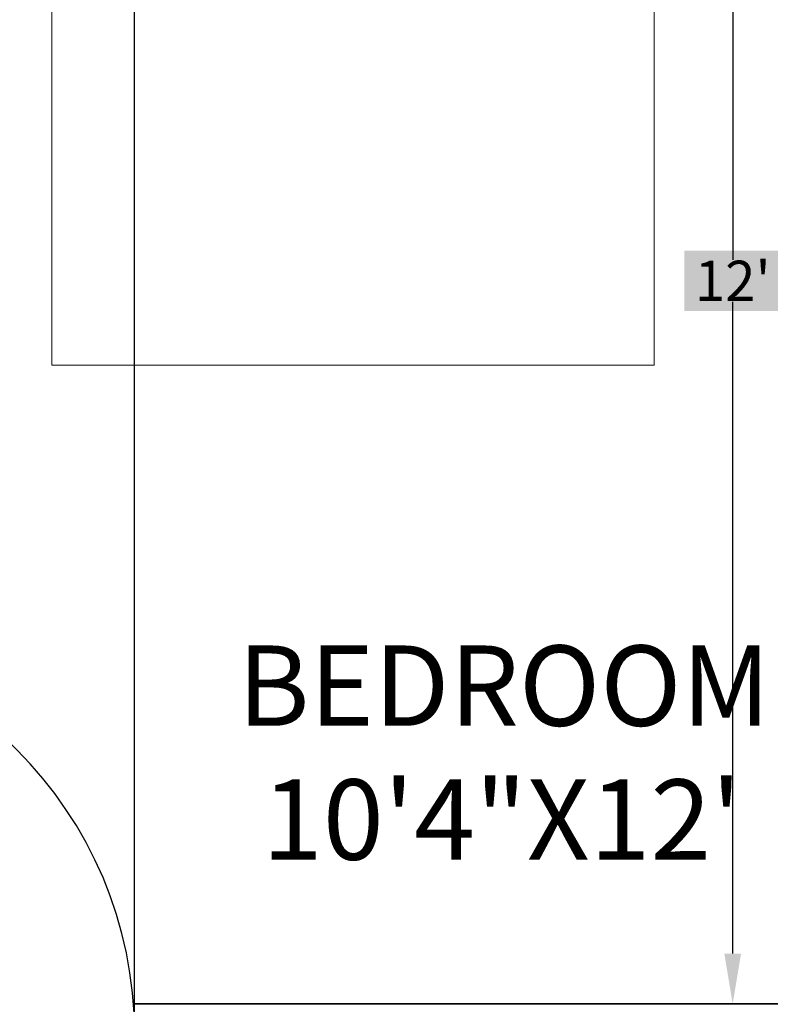
# Model space of a CAD drawing. Units: inches. Extents: x -128 to 854, y -395 to 398.
# Tile 44 of 61: x 209 to 284, y 196 to 294. Entities that reach past the tile are written whole.
import ezdxf

# ---------------------------------------------------------------- set-up
doc = ezdxf.new("R2010")
doc.units = ezdxf.units.IN
doc.header["$MEASUREMENT"] = 0
for name, color, linetype, lineweight in [('A-ANNO-DIMS', 2, 'Continuous', 18), ('A-AREA-IDEN', 1, 'Continuous', 18), ('A-DOOR', 4, 'Continuous', 25), ('A-FURN', 8, 'Continuous', 18), ('A-WALL', 4, 'Continuous', 35)]:
    doc.layers.add(name, color=color, linetype=linetype, lineweight=lineweight)
doc.styles.get("Standard").update_dxf_attribs({"font": 'arial.ttf'})
doc.dimstyles.get("Standard").update_dxf_attribs({"dimtxt": 0.18, "dimasz": 0.18, "dimexe": 0.18, "dimexo": 0.0625, "dimgap": 0.09, "dimtad": 0, "dimtih": 1, "dimtoh": 1, "dimdec": 1, "dimzin": 0, "dimdsep": 46, "dimlunit": 4, "dimtxsty": 'Standard', "dimcen": 0.09, "dimclrd": 1, "dimclre": 2, "dimclrt": 6, "dimadec": 0, "dimazin": 0, "dimtfac": 1, "dimtdec": 1, "dimtofl": 0, "dimtmove": 0, "dimatfit": 3, "dimfxl": 1, "dimtfill": 2, "dimtfillclr": 3, "dimtolj": 1, "dimtzin": 0, "dimarcsym": 0})

# ---------------------------------------------------------------- blocks, each defined once
blk = doc.blocks.new('*U3')
for p, q in [((0, 0), (0, -6)), ((40, 0), (40, -6))]:
    blk.add_line(p, q)
blk.add_lwpolyline([(0, 0), (0, 40), (1.75, 40), (1.75, 0)], close=True)
blk.add_arc((0, 0), 40, 0, 90)
blk = doc.blocks.new('Bed - Queen')
for p, q in [((0, -80.00003), (0, 0)), ((0, 0), (59.99999, 0)), ((59.99999, 0), (59.99999, -80.00003)), ((7.99999, -1.2), (28.79998, -1.2)), ((7.99999, -14.4), (7.99999, -1.2)), ((28.79998, -1.2), (28.79998, -14.4)), ((31.19999, -1.2), (51.99999, -1.2)), ((31.19999, -14.4), (31.19999, -1.2)), ((51.99999, -1.2), (51.99999, -16.4)), ((0, -14.4), (44.8, -14.4)), ((59.99999, -29.6), (44.8, -14.4)), ((44.8, -14.4), (44.8, -29.6)), ((51.99999, -16.4), (46.79936, -16.4)), ((44.8, -16.8), (0, -16.8)), ((44.8, -29.6), (59.99999, -29.6)), ((59.99999, -80.00003), (0, -80.00003))]:
    blk.add_line(p, q)
blk = doc.blocks.new('*D53')
at = {"layer": 'A-ANNO-DIMS', "color": 0, "lineweight": -2, "transparency": 16777216}
for p, q in [((304.81, 339.741), (280.297, 339.741)), ((280.477, 334.741), (280.477, 269.839)), ((280.477, 200.741), (280.477, 265.642)), ((304.81, 195.741), (280.297, 195.741))]:
    blk.add_line(p, q, dxfattribs=at)
at = {"layer": 'A-ANNO-DIMS', "color": 0, "transparency": 16777216}
for points in [[(279.644, 334.741), (281.311, 334.741), (280.477, 339.741)], [(279.644, 200.741), (281.311, 200.741), (280.477, 195.741)]]:
    blk.add_solid(points, dxfattribs=at)
at = {"layer": 'Defpoints', "color": 0, "transparency": 16777216}
for p in [(280.477, 339.741), (304.873, 339.741), (304.873, 195.741)]:
    blk.add_point(p, dxfattribs=at)
at = {"layer": 'A-ANNO-DIMS', "color": 0, "transparency": 16777216, "insert": (280.477, 267.741), "char_height": 4, "attachment_point": 5, "bg_fill": 1, "box_fill_scale": 1.25, "bg_fill_color": 3, "bg_fill_transparency": 0}
blk.add_mtext("\\A1;12'", dxfattribs=at)
blk = doc.blocks.new('*D101')
at = {"layer": 'A-ANNO-DIMS', "color": 2, "lineweight": -2, "transparency": 16777216}
for p, q in [((180.873, 186.803), (180.873, 386.743)), ((220.873, 186.803), (220.873, 386.743))]:
    blk.add_line(p, q, dxfattribs=at)
at = {"layer": 'A-ANNO-DIMS', "color": 1, "lineweight": -2, "transparency": 16777216}
for p, q in [((181.053, 386.563), (200.544, 386.563)), ((220.693, 386.563), (201.202, 386.563))]:
    blk.add_line(p, q, dxfattribs=at)
at = {"layer": 'A-ANNO-DIMS', "color": 1, "transparency": 16777216}
for points in [[(181.053, 386.593), (181.053, 386.533), (180.873, 386.563)], [(220.693, 386.593), (220.693, 386.533), (220.873, 386.563)]]:
    blk.add_solid(points, dxfattribs=at)
at = {"layer": 'Defpoints', "color": 0, "transparency": 16777216}
for p in [(220.873, 386.563), (180.873, 186.741), (220.873, 186.741)]:
    blk.add_point(p, dxfattribs=at)
at = {"layer": 'A-ANNO-DIMS', "color": 6, "transparency": 16777216, "insert": (200.873, 386.563), "char_height": 0.18, "attachment_point": 5, "bg_fill": 1, "box_fill_scale": 1.25, "bg_fill_color": 3, "bg_fill_transparency": 0}
blk.add_mtext('\\A1;3\'-4"', dxfattribs=at)

msp = doc.modelspace()

# ---------------------------------------------------------------- linework, layer by layer
at = {"layer": 'A-WALL'}
msp.add_line((304.873, 195.741), (220.76, 195.741), dxfattribs=at)

# ---------------------------------------------------------------- block references
at = {"layer": 'A-DOOR'}
msp.add_blockref('*U3', (180.873, 192.741), dxfattribs=at)
at = {"layer": 'A-FURN'}
msp.add_blockref('Bed - Queen', (212.644, 339.338), dxfattribs=at)

# ---------------------------------------------------------------- texts
at = {"layer": 'A-AREA-IDEN', "insert": (231.144, 231.425), "char_height": 8, "attachment_point": 1}
msp.add_mtext_dynamic_manual_height_columns('BEDROOM\\P 10\'4"X12\'', width=99.0352, gutter_width=1, heights=[0], dxfattribs=at)

# ---------------------------------------------------------------- dimensions: what is measured, and where the dimension line sits
at = {"layer": 'A-ANNO-DIMS'}
dim = msp.add_linear_dim(base=(220.873, 386.563), p1=(180.873, 186.741), p2=(220.873, 186.741), dimstyle='Standard', override={"dimdec": 1, "dimlfac": 1, "dimrnd": 0, "dimzin": 1, "dimdsep": 46, "dimlunit": 4, "dimfrac": 2}, dxfattribs=at)
dim.commit()
dim.dimension.update_dxf_attribs({"geometry": '*D101', "text_midpoint": (200.873, 386.563)})
dim = msp.add_linear_dim(base=(280.477, 339.741), p1=(304.873, 195.741), p2=(304.873, 339.741), angle=90, dimstyle='Standard', override={"dimtxt": 4, "dimasz": 5, "dimclrd": 0, "dimclre": 0, "dimclrt": 0}, dxfattribs=at)
dim.commit()
dim.dimension.update_dxf_attribs({"geometry": '*D53', "text_midpoint": (280.477, 267.741)})

doc.saveas('drawing.dxf')
